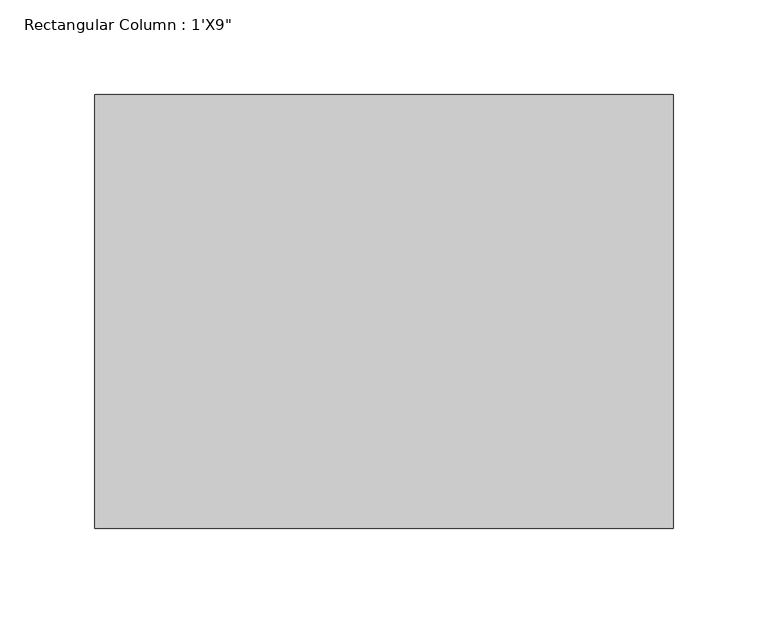
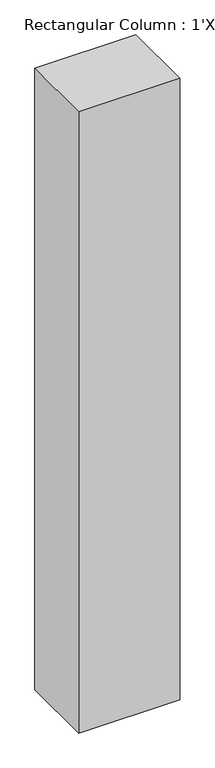
"""IFC4 building model written with IfcOpenShell, lengths in millimetres: column geometry."""

from ifc_helpers import new_model, si_unit, origin, origin_with_axes, place, context, project, spatial, polyline, outline, extrude, source, transform, mapped, element, save


def column_1646bf46(model_context):
    return source(origin(), model_context, "Body", "SweptSolid", [
        extrude(outline(polyline([(152.4, 114.3), (152.4, -114.3), (-152.4, -114.3), (-152.4, 114.3), (152.4, 114.3)])), origin_with_axes(), (0.0, 0.0, 1.0), 1981.2),
    ])


if __name__ == "__main__":
    model = new_model("IFC4")
    model_context = context("Model", 3, world=origin())
    ifc_project = project(units=[si_unit("LENGTHUNIT", "METRE", prefix="MILLI")], contexts=[model_context])
    site = spatial("IfcSite", under=ifc_project)
    building = spatial("IfcBuilding", under=site)
    placement = place(None, origin())
    column_shape = column_1646bf46(model_context)
    element("IfcColumn", 1, ObjectType="Rectangular Column : 1'X9\"", at=placement, inside=building, context=model_context, shape_type="MappedRepresentation", body=[
        mapped(column_shape, transform((0.0, 0.0, 0.0), x_axis=(1.0, 0.0, 0.0), y_axis=(0.0, 1.0, 0.0), z_axis=(0.0, 0.0, 1.0))),
    ])
    save(model, "model.ifc")

# Revit data of these elements
# Type "Rectangular Column : 1'X9\""
#   Assembly Code = "B1010200"
#   Depth = 0' - 9"
#   Offset Base = 0' - 0"
#   Offset Top = 0' - 0"
#   Width = 1' - 0"
#   Material = none
